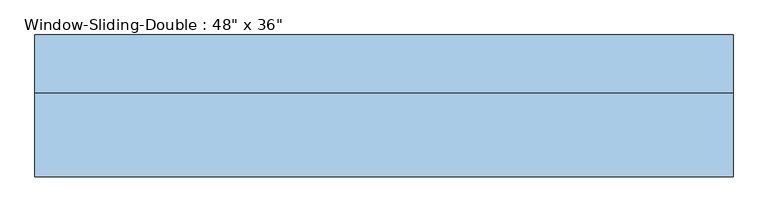
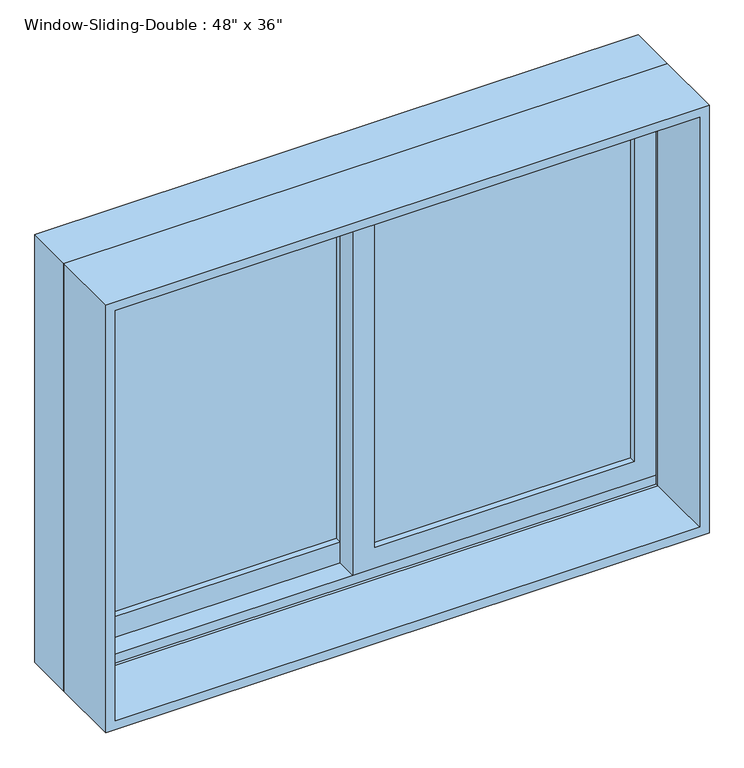
"""IFC4 building model written with IfcOpenShell, lengths in millimetres: window geometry."""

from ifc_helpers import new_model, si_unit, frame, origin, place, context, project, spatial, polyline, outline, extrude, faceted_brep, source, transform, mapped, element, save


def window_2eef0573(model_context):
    return source(origin(), model_context, "Body", "SolidModel", [
        extrude(outline(polyline([(952.5, 590.55), (1809.75, 590.55), (1809.75, -22.225), (952.5, -22.225), (952.5, 590.55)]), holes=[polyline([(996.95, 22.225), (1765.3, 22.225), (1765.3, 546.1), (996.95, 546.1), (996.95, 22.225)])]), frame((0.0, 34.29, 0.0), z_axis=(0.0, 1.0, 0.0), x_axis=(0.0, 0.0, 1.0)), (0.0, 0.0, 1.0), 44.45),
        extrude(outline(polyline([(933.45, -590.55), (933.45, 22.225), (1809.75, 22.225), (1809.75, -590.55), (933.45, -590.55)]), holes=[polyline([(1765.3, -22.225), (996.95, -22.225), (996.95, -546.1), (1765.3, -546.1), (1765.3, -22.225)])]), frame((0.0, 78.74, 0.0), z_axis=(0.0, 1.0, 0.0), x_axis=(0.0, 0.0, 1.0)), (0.0, 0.0, 1.0), 44.45),
        extrude(outline(polyline([(-22.225, 110.49), (-22.225, 104.14), (-546.1, 104.14), (-546.1, 110.49), (-22.225, 110.49)])), frame((0.0, 0.0, 996.95), z_axis=(0.0, 0.0, 1.0), x_axis=(1.0, 0.0, 0.0)), (0.0, 0.0, 1.0), 768.35),
        extrude(outline(polyline([(-22.225, 97.79), (-22.225, 91.44), (-546.1, 91.44), (-546.1, 97.79), (-22.225, 97.79)])), frame((0.0, 0.0, 996.95), z_axis=(0.0, 0.0, 1.0), x_axis=(1.0, 0.0, 0.0)), (0.0, 0.0, 1.0), 768.35),
        extrude(outline(polyline([(546.1, 66.04), (546.1, 59.69), (22.225, 59.69), (22.225, 66.04), (546.1, 66.04)])), frame((0.0, 0.0, 996.95), z_axis=(0.0, 0.0, 1.0), x_axis=(1.0, 0.0, 0.0)), (0.0, 0.0, 1.0), 768.35),
        extrude(outline(polyline([(546.1, 53.34), (546.1, 46.99), (22.225, 46.99), (22.225, 53.34), (546.1, 53.34)])), frame((0.0, 0.0, 996.95), z_axis=(0.0, 0.0, 1.0), x_axis=(1.0, 0.0, 0.0)), (0.0, 0.0, 1.0), 768.35),
        extrude(outline(polyline([(1828.8, -609.6), (914.4, -609.6), (914.4, 609.6), (1828.8, 609.6), (1828.8, -609.6)]), holes=[polyline([(1809.75, 590.55), (933.45, 590.55), (933.45, -590.55), (1809.75, -590.55), (1809.75, 590.55)])]), frame((0.0, -118.11, 0.0), z_axis=(0.0, 1.0, 0.0), x_axis=(0.0, 0.0, 1.0)), (0.0, 0.0, 1.0), 146.05),
        faceted_brep([(-609.6, 27.94, 914.4), (-609.6, 129.54, 914.4), (609.6, 129.54, 914.4), (609.6, 27.94, 914.4), (-568.6778905, 129.54, 1787.8778905), (-568.6778905, 123.19, 1787.8778905), (-568.6778905, 123.19, 933.45), (-568.6778905, 129.54, 933.45), (568.6778905, 123.19, 1787.8778905), (568.6778905, 123.19, 933.45), (590.55, 123.19, 933.45), (590.55, 123.19, 1809.75), (-590.55, 123.19, 1809.75), (-590.55, 123.19, 933.45), (-590.55, 27.94, 1809.75), (-590.55, 27.94, 933.45), (-590.55, 34.29, 933.45), (-590.55, 34.29, 952.5), (-590.55, 78.74, 952.5), (-590.55, 78.74, 933.45), (609.6, 27.94, 1828.8), (-609.6, 27.94, 1828.8), (590.55, 27.94, 1809.75), (590.55, 27.94, 933.45), (-609.6, 129.54, 1828.8), (609.6, 129.54, 1828.8), (568.6778905, 129.54, 933.45), (568.6778905, 129.54, 1787.8778905), (590.55, 78.74, 933.45), (590.55, 78.74, 952.5), (590.55, 34.29, 952.5), (590.55, 34.29, 933.45)], [[[0, 1, 2, 3]], [[4, 5, 6, 7]], [[5, 8, 9, 10, 11, 12, 13, 6]], [[12, 14, 15, 16, 17, 18, 19, 13]], [[0, 3, 20, 21], [22, 23, 15, 14]], [[24, 1, 0, 21]], [[2, 1, 24, 25], [4, 7, 26, 27]], [[5, 4, 27, 8]], [[12, 11, 22, 14]], [[21, 20, 25, 24]], [[8, 27, 26, 9]], [[22, 11, 10, 28, 29, 30, 31, 23]], [[20, 3, 2, 25]], [[26, 7, 6, 13, 19, 28, 10, 9]], [[28, 19, 18, 29]], [[29, 18, 17, 30]], [[30, 17, 16, 31]], [[15, 23, 31, 16]]]),
    ])


if __name__ == "__main__":
    model = new_model("IFC4")
    model_context = context("Model", 3, world=origin())
    ifc_project = project(units=[si_unit("LENGTHUNIT", "METRE", prefix="MILLI")], contexts=[model_context])
    site = spatial("IfcSite", under=ifc_project)
    building = spatial("IfcBuilding", under=site)
    placement = place(None, origin())
    window_shape = window_2eef0573(model_context)
    element("IfcWindow", 1, ObjectType="Window-Sliding-Double : 48\" x 36\"", at=placement, inside=building, context=model_context, shape_type="MappedRepresentation", body=[
        mapped(window_shape, transform((0.0, 0.0, 0.0), x_axis=(1.0, 0.0, 0.0), y_axis=(0.0, 1.0, 0.0), z_axis=(0.0, 0.0, 1.0))),
    ])
    save(model, "model.ifc")

# Revit data of these elements
# Type "Window-Sliding-Double : 48\" x 36\""
#   Type Mark = "20"
#   Fire Rating = "0.5h"
#   Assembly Code = "B2020100"
#   Analytic Construction = "Double glazing - domestic"
#   Window Inset [instance default] = 0' - 0"
#   Wall Thickness [instance default] = 0' - 6"
#   Visual Light Transmittance = 0.81
#   Thermal Resistance (R) = 1.8146 (h·ft²·°F)/BTU
#   Solar Heat Gain Coefficient = 0.76
#   Muntin Width = 1' - 8 5/8"
#   Muntin Height = 2' - 6 1/4"
#   Interior Wall Closure [instance default] = 0' - 2 3/4"
#   Heat Transfer Coefficient (U) = 0.5511 BTU/(h·ft²·°F)
#   Frame Extension [instance default] = 0' - 0 1/4"
#   Exterior Wall Closure [instance default] = 0' - 1 1/4"
#   Rough Width = 4' - 0 1/2"
#   Rough Height = 3' - 0 1/2"
#   Height = 3' - 0"
#   Extension Jamb [instance default] = 0' - 2 3/4"
#   Default Sill Height = 3' - 0"
#   Width = 4' - 0"
#   Interior Trim Visibility [instance default] = yes
#   Indicator Visibility [instance default] = yes
#   Exterior Trim Visibility [instance default] = yes
#   Muntin Visibility = yes
#   Extension Jamb Visibility [instance default] = yes
#   Muntin Pattern = Muntin Pattern_2x2 : Muntin Pattern_2x2
#   Interior Trim Material = Wood - Stained
#   Interior Trim = Trim-Window-Interior-Flat : Picture Frame
#   Interior Frame Material = Wood - Stained
#   Glass Panel Material = Glass
#   Exterior Trim Material = Clad - White
#   Exterior Trim = Trim-Window-Exterior-Flat : with Sill
#   Exterior Frame Material = Clad - White
#   Wall Closure = (empty or 0)
# Element 1 (IfcWindow, "Window-Sliding-Double : 48\" x 36\"")
#   Wall Thickness = 0' - 9"
#   Extension Jamb = 0' - 5 3/4"
#   Materials on its faces: "Wood - Stained", "Glass", "Clad - White"
# Materials
#   "Wood - Stained": class "Wood", colour RGB 224 178 126, transparency 0, Cost = 0
#   "Glass": class "Glass", colour RGB 0 128 192, transparency 0.75, Description = "Soda Lime Glass", Cost = 0
#   "Clad - White": class "Wood", colour RGB 242 242 238, transparency 0, Cost = 0
